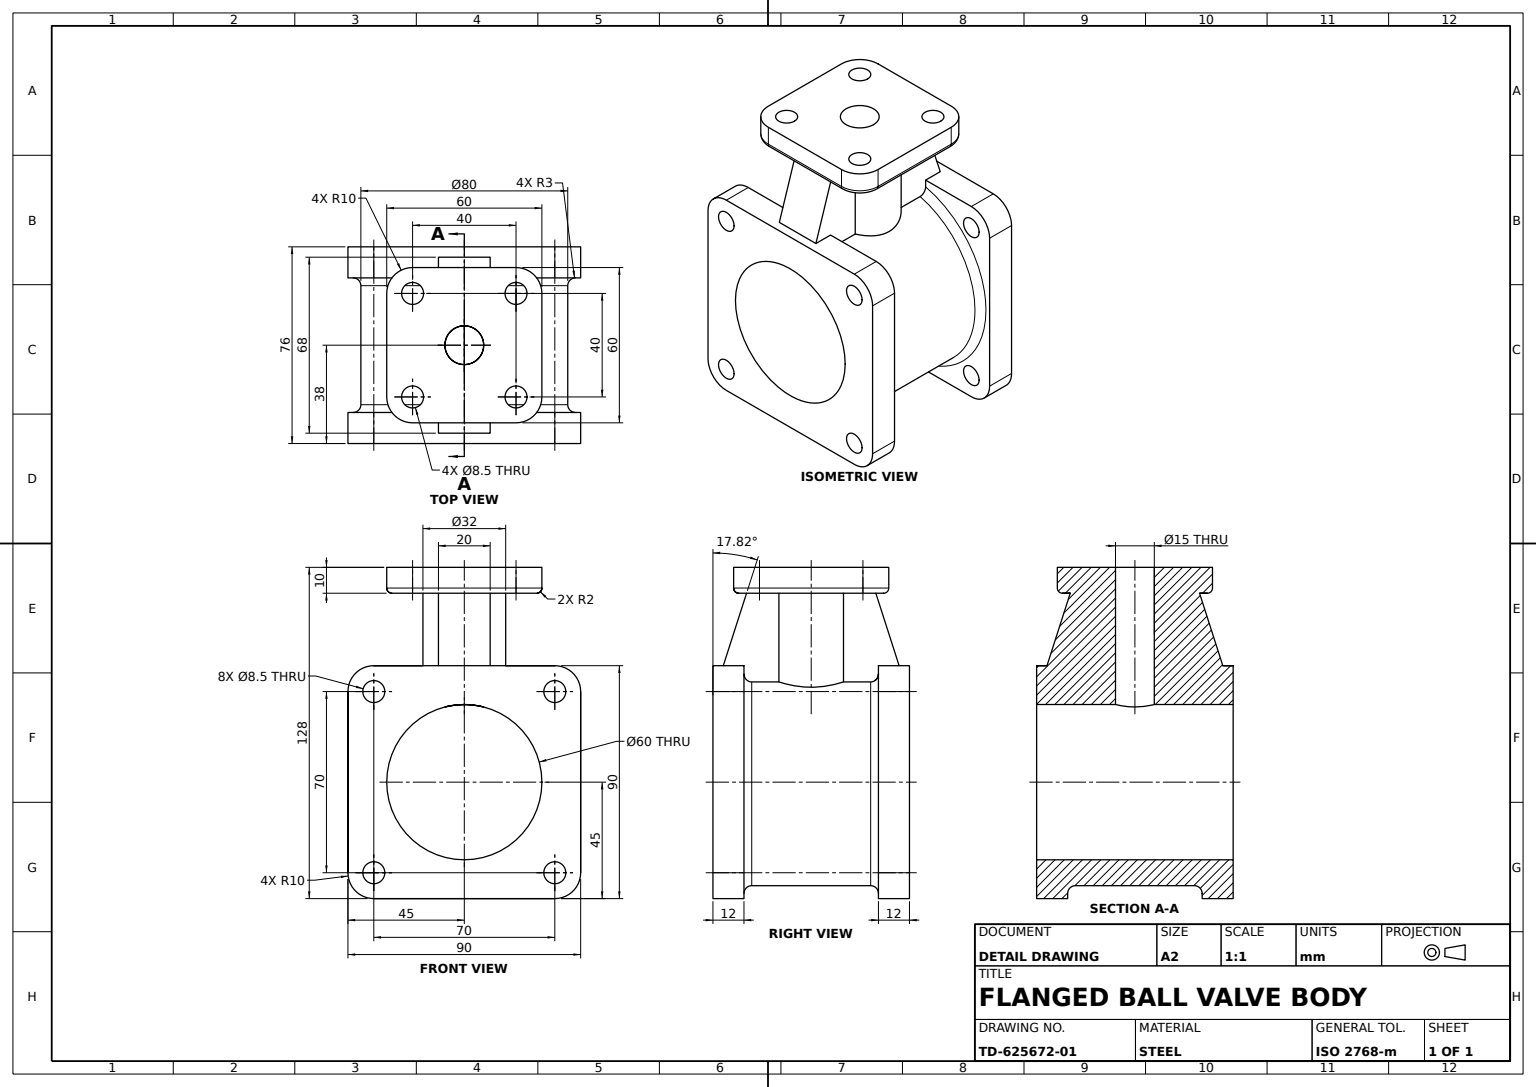
from build123d import *

# Parameters (mm, degrees)
BODY_TUBE_SKETCH_R                 = 40
BODY_TUBE_SKETCH_R_2               = 30
BODY_TUBE_DEPTH                    = 76
END_FLANGE_DEPTH                   = 12
BODY_BORE_SKETCH_R                 = 30
BODY_BORE_60_DEPTH                 = 100.126182212
END_FLANGE_BOLT_HOLES_SKETCH_R     = 4.25
END_FLANGE_BOLT_HOLES_4X_8_5_DEPTH = 12
TOP_FLANGE_DEPTH                   = 10
STEM_NECK_SKETCH_R                 = 16
STEM_NECK_32_DEPTH                 = 48
NECK_SUPPORT_RIB_DEPTH             = 10
TOP_FLANGE_BOLT_HOLES_SKETCH_R     = 4.25
TOP_FLANGE_BOLT_HOLES_4X_8_5_DEPTH = 20
STEM_BORE_SKETCH_R                 = 7.5
STEM_BORE_15_DEPTH                 = 54
END_FLANGE_FILLETS_R3_R            = 3
TOP_FLANGE_FILLETS_R2_R            = 2


with BuildPart() as part:
    # Body Tube Sketch → Body Tube (new body)
    with BuildSketch(Plane(origin=(0, 0, 0), x_dir=(0, 0, -1), z_dir=(1, 0, 0))):
        Circle(BODY_TUBE_SKETCH_R)
        Circle(BODY_TUBE_SKETCH_R_2, mode=Mode.SUBTRACT)
    extrude(amount=BODY_TUBE_DEPTH)

    # End Flange Sketch → End Flange (add)
    with BuildSketch(Plane.ZY):
        with BuildLine():
            Line((-35, -45), (35, -45))
            ThreePointArc((35, -45), (42.071067812, -42.071067812), (45, -35))
            Line((45, -35), (45, 35))
            ThreePointArc((45, 35), (42.071067812, 42.071067812), (35, 45))
            Line((35, 45), (-35, 45))
            ThreePointArc((-35, 45), (-42.071067812, 42.071067812), (-45, 35))
            Line((-45, 35), (-45, -35))
            ThreePointArc((-45, -35), (-42.071067812, -42.071067812), (-35, -45))
        make_face()
    end_flange = extrude(amount=-END_FLANGE_DEPTH)

    # Body Bore Sketch → Body Bore Ø60 (cut, through all)
    with BuildSketch(Plane.ZY):
        Circle(BODY_BORE_SKETCH_R)
    body_bore_60 = extrude(amount=-BODY_BORE_60_DEPTH, mode=Mode.SUBTRACT)

    # End Flange Bolt Holes Sketch → End Flange Bolt Holes 4xØ8.5 (cut)
    with BuildSketch(Plane.ZY):
        with Locations((-35, 35)):
            Circle(END_FLANGE_BOLT_HOLES_SKETCH_R)
        with Locations((35, 35)):
            Circle(END_FLANGE_BOLT_HOLES_SKETCH_R)
        with Locations((-35, -35)):
            Circle(END_FLANGE_BOLT_HOLES_SKETCH_R)
        with Locations((35, -35)):
            Circle(END_FLANGE_BOLT_HOLES_SKETCH_R)
    end_flange_bolt_holes_4x_8_5 = extrude(amount=-END_FLANGE_BOLT_HOLES_4X_8_5_DEPTH, mode=Mode.SUBTRACT)

    # Opposite End Flange Mirror: End Flange across plane
    add(end_flange.mirror(Plane(origin=(38, 0, 0), x_dir=(0, 0, 1), z_dir=(1, 0, 0))))

    # Opposite Flange Holes and Bore Mirror: Body Bore Ø60, End Flange Bolt Holes 4xØ8.5 across plane
    add(body_bore_60.mirror(Plane(origin=(38, 0, 0), x_dir=(0, 0, 1), z_dir=(1, 0, 0))), mode=Mode.SUBTRACT)
    add(end_flange_bolt_holes_4x_8_5.mirror(Plane(origin=(38, 0, 0), x_dir=(0, 0, 1), z_dir=(1, 0, 0))), mode=Mode.SUBTRACT)



with BuildPart() as body_2:
    # Top Flange Sketch → Top Flange (new body)
    with BuildSketch(Plane(origin=(0, 83, 0), x_dir=(1, 0, 0), z_dir=(0, 1, 0))):
        with BuildLine():
            Line((18, -30), (58, -30))
            ThreePointArc((58, -30), (65.071067812, -27.071067812), (68, -20))
            Line((68, -20), (68, 20))
            ThreePointArc((68, 20), (65.071067812, 27.071067812), (58, 30))
            Line((58, 30), (18, 30))
            ThreePointArc((18, 30), (10.928932188, 27.071067812), (8, 20))
            Line((8, 20), (8, -20))
            ThreePointArc((8, -20), (10.928932188, -27.071067812), (18, -30))
        make_face()
    extrude(amount=-TOP_FLANGE_DEPTH)


with BuildPart() as part_1:
    add(part.part)

    add(body_2.part)  # Stem Neck Ø32 merges body 2
    # Stem Neck Sketch → Stem Neck Ø32 (add)
    with BuildSketch(Plane(origin=(0, 83, 0), x_dir=(1, 0, 0), z_dir=(0, 1, 0))):
        with Locations(Location((38, 0, 0), (0, 0, 270))):
            Circle(STEM_NECK_SKETCH_R)
    extrude(amount=-STEM_NECK_32_DEPTH)

    # Neck Support Rib Sketch → Neck Support Rib (add, symmetric)
    with BuildSketch(Plane.XY):
        Polygon((27.229131896, 73), (27.229131896, 33), (12, 33), (12, 45), (4, 45), (13, 73), align=None)
    neck_support_rib = extrude(amount=NECK_SUPPORT_RIB_DEPTH, both=True)

    # Neck Support Rib Mirror: Neck Support Rib across plane
    add(neck_support_rib.mirror(Plane(origin=(38, 0, 0), x_dir=(0, 0, 1), z_dir=(1, 0, 0))))

    # Top Flange Bolt Holes Sketch → Top Flange Bolt Holes 4xØ8.5 (cut)
    with BuildSketch(Plane(origin=(0, 83, 0), x_dir=(1, 0, 0), z_dir=(0, 1, 0))):
        with Locations(Location((18, 20, 0), (0, 0, 270))):
            Circle(TOP_FLANGE_BOLT_HOLES_SKETCH_R)
        with Locations(Location((58, 20, 0), (0, 0, 270))):
            Circle(TOP_FLANGE_BOLT_HOLES_SKETCH_R)
        with Locations(Location((18, -20, 0), (0, 0, 270))):
            Circle(TOP_FLANGE_BOLT_HOLES_SKETCH_R)
        with Locations(Location((58, -20, 0), (0, 0, 270))):
            Circle(TOP_FLANGE_BOLT_HOLES_SKETCH_R)
    extrude(amount=-TOP_FLANGE_BOLT_HOLES_4X_8_5_DEPTH, mode=Mode.SUBTRACT)

    # Stem Bore Sketch → Stem Bore Ø15 (cut)
    with BuildSketch(Plane(origin=(0, 83, 0), x_dir=(1, 0, 0), z_dir=(0, 1, 0))):
        with Locations(Location((38, 0, 0), (0, 0, 270))):
            Circle(STEM_BORE_SKETCH_R)
    extrude(amount=-STEM_BORE_15_DEPTH, mode=Mode.SUBTRACT)

    # End Flange Fillets R3
    end_flange_fillets_r3_edges = [part_1.edges().sort_by_distance(p)[0] for p in [
        (12, -31.622776602, 24.494897428),
        (64, -31.622776602, 24.494897428),
    ]]
    fillet(end_flange_fillets_r3_edges, radius=END_FLANGE_FILLETS_R3_R)

    # Top Flange Fillets R2
    top_flange_fillets_r2_edges = [part_1.edges().sort_by_distance(p)[0] for p in [
        (10.928932188, 73, 27.071067812),
        (8, 73, 0),
        (10.928932188, 73, -27.071067812),
        (38, 73, -30),
        (65.071067812, 73, -27.071067812),
        (68, 73, 0),
        (65.071067812, 73, 27.071067812),
        (38, 73, 30),
    ]]
    fillet(top_flange_fillets_r2_edges, radius=TOP_FLANGE_FILLETS_R2_R)


solid = part_1.part
